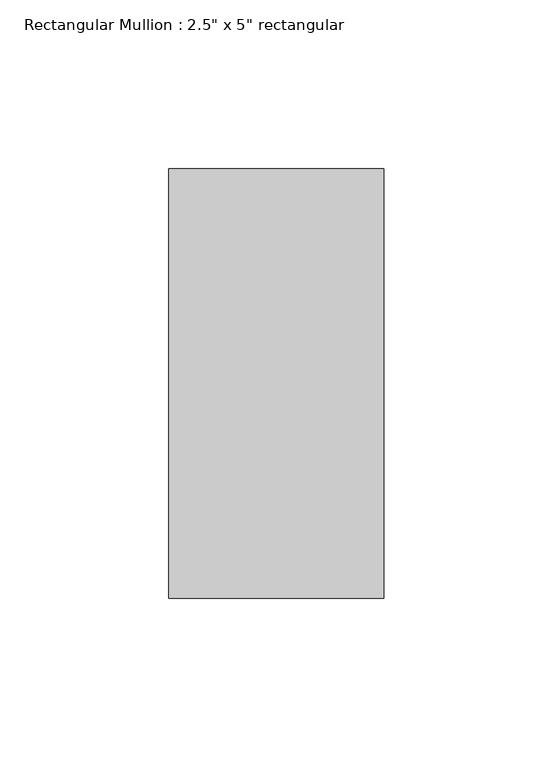
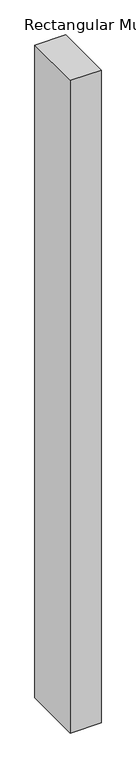
"""IFC4 building model written with IfcOpenShell, lengths in millimetres: member geometry."""

from ifc_helpers import new_model, si_unit, frame, origin, place, context, project, spatial, polyline, outline, extrude, source, transform, mapped, element, save


def member_5493b72c(model_context):
    return source(origin(), model_context, "Body", "SweptSolid", [
        extrude(outline(polyline([(0.0, 63.5), (0.0, -63.5), (-63.5, -63.5), (-63.5, 63.5), (0.0, 63.5)])), frame((0.0, 0.0, -1428.1991558), z_axis=(0.0, 0.0, 1.0), x_axis=(1.0, 0.0, 0.0)), (0.0, 0.0, 1.0), 1428.1991558),
    ])


if __name__ == "__main__":
    model = new_model("IFC4")
    model_context = context("Model", 3, world=origin())
    ifc_project = project(units=[si_unit("LENGTHUNIT", "METRE", prefix="MILLI")], contexts=[model_context])
    site = spatial("IfcSite", under=ifc_project)
    building = spatial("IfcBuilding", under=site)
    placement = place(None, origin())
    member_shape = member_5493b72c(model_context)
    element("IfcMember", 1, ObjectType="Rectangular Mullion : 2.5\" x 5\" rectangular", at=placement, inside=building, context=model_context, shape_type="MappedRepresentation", body=[
        mapped(member_shape, transform((0.0, 0.0, 0.0), x_axis=(1.0, 0.0, 0.0), y_axis=(0.0, 1.0, 0.0), z_axis=(0.0, 0.0, 1.0))),
    ])
    save(model, "model.ifc")

# Revit data of these elements
# Type "Rectangular Mullion : 2.5\" x 5\" rectangular"
#   built-in parameter 1007304 = 0.416667 (stored number, unit not read)
#   built-in parameter 1007301 = 0.104167 (stored number, unit not read)
#   built-in parameter 1007300 = 0.104167 (stored number, unit not read)
# Element 1 (IfcMember, "Rectangular Mullion : 2.5\" x 5\" rectangular")
#   Materials on its faces: "Aluminum"
# Materials
#   "Aluminum": class "Metal", colour RGB 247 247 247, transparency 0, Description = "Aluminum 6061", Cost = 0
